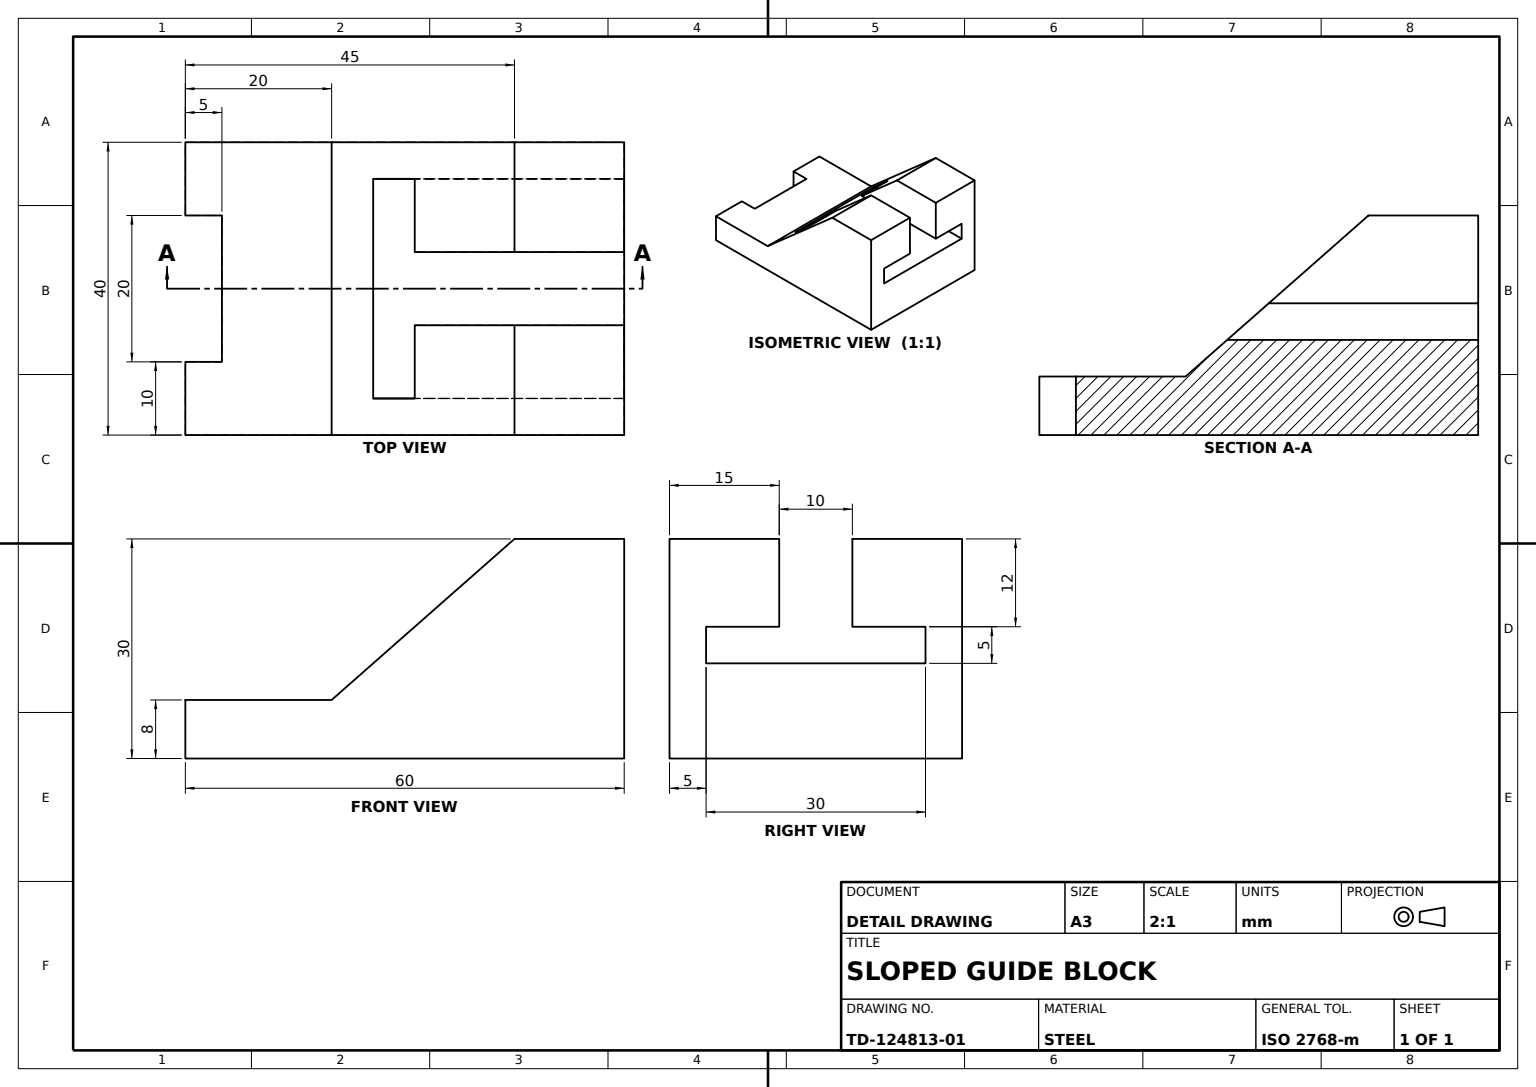
from build123d import *

# Parameters (mm, degrees)
ANGLED_BASE_BLOCK_DEPTH  = 40
GROOVE_CUT_5MM_DEPTH     = 5
T_SLOT_THROUGH_CUT_DEPTH = 40


with BuildPart() as part:
    # Base Profile Sketch → Angled Base Block (new body)
    with BuildSketch(Plane.XY):
        Polygon((0, 0), (60, 0), (60, 30), (45, 30), (20, 8), (0, 8), align=None)
    extrude(amount=ANGLED_BASE_BLOCK_DEPTH)

    # Groove Profile Sketch → Groove Cut 5mm (cut)
    with BuildSketch(Plane.ZY):
        Polygon((20, 8), (10, 8), (10, 0), (30, 0), (30, 8), align=None)
    extrude(amount=-GROOVE_CUT_5MM_DEPTH, mode=Mode.SUBTRACT)

    # T-Slot Profile Sketch → T-Slot Through Cut (cut)
    with BuildSketch(Plane(origin=(60, 0, 0), x_dir=(0, 0, -1), z_dir=(1, 0, 0))):
        Polygon((-20, 30), (-25, 30), (-25, 18), (-35, 18), (-35, 13), (-5, 13), (-5, 18), (-15, 18), (-15, 30), align=None)
    extrude(amount=-T_SLOT_THROUGH_CUT_DEPTH, mode=Mode.SUBTRACT)


solid = part.part
